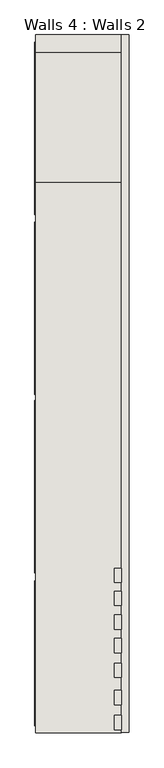
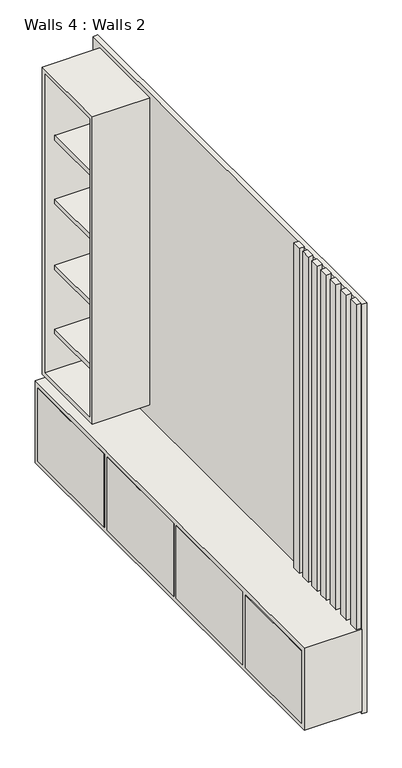
"""IFC4 building model written with IfcOpenShell, lengths in millimetres: wall geometry, Walls 4 : Walls 2."""

from ifc_helpers import new_model, si_unit, frame, origin, place, context, project, spatial, polyline, outline, extrude, faceted_brep, source, transform, mapped, element, save


def walls_4_walls_2_ccd45d7e(model_context):
    return source(origin(), model_context, "Body", "SolidModel", [
        extrude(outline(polyline([(-1167.1478577, -3563.611411), (-1167.1478577, -3052.3039411), (-1164.5681702, -3052.3039411), (-1164.5681702, -3563.611411), (-1167.1478577, -3563.611411)])), frame((0.0, 0.0, 3240.532709), z_axis=(0.0, 0.0, 1.0), x_axis=(1.0, 0.0, 0.0)), (0.0, 0.0, 1.0), 406.4),
        extrude(outline(polyline([(-1167.1478577, -3023.861411), (-1167.1478577, -2414.261411), (-1164.5681702, -2414.261411), (-1164.5681702, -3023.861411), (-1167.1478577, -3023.861411)])), frame((0.0, 0.0, 3240.532709), z_axis=(0.0, 0.0, 1.0), x_axis=(1.0, 0.0, 0.0)), (0.0, 0.0, 1.0), 406.4),
        extrude(outline(polyline([(-1167.1478577, -2393.557676), (-1167.1478577, -1783.957676), (-1164.5681702, -1783.957676), (-1164.5681702, -2393.557676), (-1167.1478577, -2393.557676)])), frame((0.0, 0.0, 3240.532709), z_axis=(0.0, 0.0, 1.0), x_axis=(1.0, 0.0, 0.0)), (0.0, 0.0, 1.0), 406.4),
        extrude(outline(polyline([(-1167.1478577, -1758.557676), (-1167.1478577, -1148.957676), (-1164.5681702, -1148.957676), (-1164.5681702, -1758.557676), (-1167.1478577, -1758.557676)])), frame((0.0, 0.0, 3240.532709), z_axis=(0.0, 0.0, 1.0), x_axis=(1.0, 0.0, 0.0)), (0.0, 0.0, 1.0), 406.4),
        extrude(outline(polyline([(-885.1681702, -3577.3260888), (-885.1681702, -3526.5260888), (-859.7681702, -3526.5260888), (-859.7681702, -3577.3260888), (-885.1681702, -3577.3260888)])), frame((0.0, 0.0, 3672.332709), z_axis=(0.0, 0.0, 1.0), x_axis=(1.0, 0.0, 0.0)), (0.0, 0.0, 1.0), 1815.6625633),
        extrude(outline(polyline([(-885.1681702, -3489.4392633), (-885.1681702, -3438.6392633), (-859.7681702, -3438.6392633), (-859.7681702, -3489.4392633), (-885.1681702, -3489.4392633)])), frame((0.0, 0.0, 3672.332709), z_axis=(0.0, 0.0, 1.0), x_axis=(1.0, 0.0, 0.0)), (0.0, 0.0, 1.0), 1815.6625633),
        extrude(outline(polyline([(-885.1681702, -3222.7392633), (-885.1681702, -3171.9392633), (-859.7681702, -3171.9392633), (-859.7681702, -3222.7392633), (-885.1681702, -3222.7392633)])), frame((0.0, 0.0, 3672.332709), z_axis=(0.0, 0.0, 1.0), x_axis=(1.0, 0.0, 0.0)), (0.0, 0.0, 1.0), 1815.6625633),
        extrude(outline(polyline([(-885.1681702, -3393.1760888), (-885.1681702, -3342.3760888), (-859.7681702, -3342.3760888), (-859.7681702, -3393.1760888), (-885.1681702, -3393.1760888)])), frame((0.0, 0.0, 3672.332709), z_axis=(0.0, 0.0, 1.0), x_axis=(1.0, 0.0, 0.0)), (0.0, 0.0, 1.0), 1815.6625633),
        extrude(outline(polyline([(-885.1681702, -3305.2892633), (-885.1681702, -3254.4892633), (-859.7681702, -3254.4892633), (-859.7681702, -3305.2892633), (-885.1681702, -3305.2892633)])), frame((0.0, 0.0, 3672.332709), z_axis=(0.0, 0.0, 1.0), x_axis=(1.0, 0.0, 0.0)), (0.0, 0.0, 1.0), 1815.6625633),
        extrude(outline(polyline([(-885.1681702, -3139.1760888), (-885.1681702, -3088.3760888), (-859.7681702, -3088.3760888), (-859.7681702, -3139.1760888), (-885.1681702, -3139.1760888)])), frame((0.0, 0.0, 3672.332709), z_axis=(0.0, 0.0, 1.0), x_axis=(1.0, 0.0, 0.0)), (0.0, 0.0, 1.0), 1815.6625633),
        extrude(outline(polyline([(-885.1681702, -3057.9595435), (-885.1681702, -3007.1595435), (-859.7681702, -3007.1595435), (-859.7681702, -3057.9595435), (-885.1681702, -3057.9595435)])), frame((0.0, 0.0, 3672.332709), z_axis=(0.0, 0.0, 1.0), x_axis=(1.0, 0.0, 0.0)), (0.0, 0.0, 1.0), 1815.6625633),
        extrude(outline(polyline([(-1164.5681702, -3587.357676), (-1164.5681702, -1123.557676), (-859.7681702, -1123.557676), (-859.7681702, -3587.357676), (-1164.5681702, -3587.357676)])), frame((0.0, 0.0, 3215.132709), z_axis=(0.0, 0.0, 1.0), x_axis=(1.0, 0.0, 0.0)), (0.0, 0.0, 1.0), 457.2),
        extrude(outline(polyline([(-1113.7681702, -1618.857676), (-1113.7681702, -1212.457676), (-885.1681702, -1212.457676), (-885.1681702, -1618.857676), (-1113.7681702, -1618.857676)])), frame((0.0, 0.0, 5052.8679591), z_axis=(0.0, 0.0, 1.0), x_axis=(1.0, 0.0, 0.0)), (0.0, 0.0, 1.0), 25.4),
        extrude(outline(polyline([(-1113.7681702, -1618.857676), (-1113.7681702, -1212.457676), (-885.1681702, -1212.457676), (-885.1681702, -1618.857676), (-1113.7681702, -1618.857676)])), frame((0.0, 0.0, 4697.2679591), z_axis=(0.0, 0.0, 1.0), x_axis=(1.0, 0.0, 0.0)), (0.0, 0.0, 1.0), 25.4),
        extrude(outline(polyline([(-1113.7681702, -1618.857676), (-1113.7681702, -1212.457676), (-885.1681702, -1212.457676), (-885.1681702, -1618.857676), (-1113.7681702, -1618.857676)])), frame((0.0, 0.0, 4328.9679591), z_axis=(0.0, 0.0, 1.0), x_axis=(1.0, 0.0, 0.0)), (0.0, 0.0, 1.0), 25.4),
        extrude(outline(polyline([(-1113.7681702, -1618.857676), (-1113.7681702, -1212.457676), (-885.1681702, -1212.457676), (-885.1681702, -1618.857676), (-1113.7681702, -1618.857676)])), frame((0.0, 0.0, 3971.9696931), z_axis=(0.0, 0.0, 1.0), x_axis=(1.0, 0.0, 0.0)), (0.0, 0.0, 1.0), 25.4),
        faceted_brep([(-1164.5681702, -1644.257676, 5462.5952722), (-1164.5681702, -1187.057676, 5462.5952722), (-1164.5681702, -1187.057676, 3746.39238), (-1164.5681702, -1644.257676, 3746.39238), (-1164.5681702, -1618.857676, 5437.1952722), (-1164.5681702, -1618.857676, 3771.79238), (-1164.5681702, -1212.457676, 3771.79238), (-1164.5681702, -1212.457676, 5437.1952722), (-859.7681702, -1644.257676, 5462.5952722), (-859.7681702, -1644.257676, 3746.39238), (-859.7681702, -1187.057676, 3746.39238), (-859.7681702, -1187.057676, 5462.5952722), (-885.1681702, -1618.857676, 5437.1952722), (-885.1681702, -1212.457676, 5437.1952722), (-885.1681702, -1212.457676, 3771.79238), (-885.1681702, -1618.857676, 3771.79238)], [[[0, 1, 2, 3], [4, 5, 6, 7]], [[8, 9, 10, 11]], [[1, 0, 8, 11]], [[2, 1, 11, 10]], [[3, 2, 10, 9]], [[0, 3, 9, 8]], [[12, 13, 14, 15]], [[12, 15, 5, 4]], [[15, 14, 6, 5]], [[14, 13, 7, 6]], [[13, 12, 4, 7]]]),
        extrude(outline(polyline([(-859.7681702, -3587.357676), (-859.7681702, -1123.557676), (-834.3681702, -1123.557676), (-834.3681702, -3587.357676), (-859.7681702, -3587.357676)])), frame((0.0, 0.0, 3200.4), z_axis=(0.0, 0.0, 1.0), x_axis=(1.0, 0.0, 0.0)), (0.0, 0.0, 1.0), 2287.5952722),
    ])


if __name__ == "__main__":
    model = new_model("IFC4")
    model_context = context("Model", 3, world=origin())
    ifc_project = project(units=[si_unit("LENGTHUNIT", "METRE", prefix="MILLI")], contexts=[model_context])
    site = spatial("IfcSite", under=ifc_project)
    building = spatial("IfcBuilding", under=site)
    placement = place(None, origin())
    walls_4_walls_2_shape = walls_4_walls_2_ccd45d7e(model_context)
    element("IfcWall", 1, ObjectType="Walls 4 : Walls 2", at=placement, inside=building, context=model_context, shape_type="MappedRepresentation", body=[
        mapped(walls_4_walls_2_shape, transform((0.0, 0.0, 0.0), x_axis=(1.0, 0.0, 0.0), y_axis=(0.0, 1.0, 0.0), z_axis=(0.0, 0.0, 1.0))),
    ])
    save(model, "model.ifc")

# Revit data of these elements
# Element 1 (IfcWall, "Walls 4 : Walls 2")
#   Materials on its faces: "drawers", "metal", "wood"
# Materials
#   "drawers": class "Generic", colour RGB 121 66 39, transparency 0, Cost = 0
#   "metal": class "Generic", colour RGB 76 25 7, transparency 0, Cost = 0
#   "wood": class "Generic", colour RGB 255 226 181, transparency 0, Cost = 0
